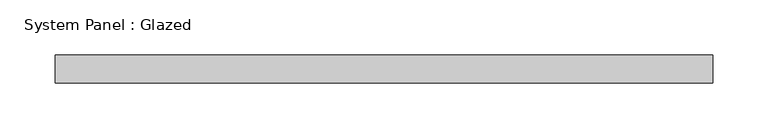
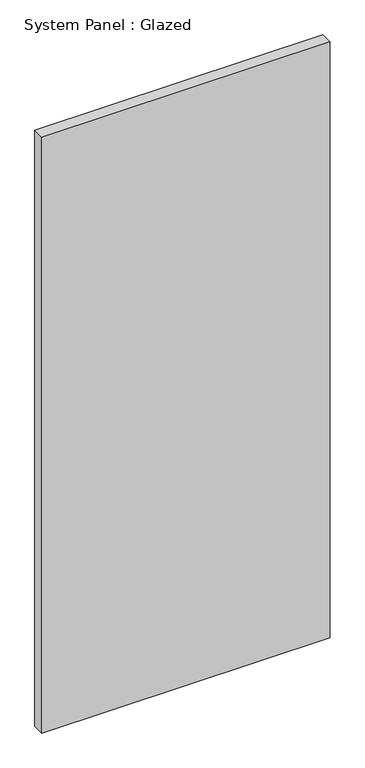
"""IFC4 building model written with IfcOpenShell, lengths in millimetres: plate geometry, System Panel : Glazed."""

from ifc_helpers import new_model, si_unit, origin, origin_with_axes, place, context, project, spatial, polyline, outline, extrude, source, transform, mapped, element, save


def system_panel_glazed_01fedee4(model_context):
    return source(origin(), model_context, "Body", "SweptSolid", [
        extrude(outline(polyline([(298.45, 19.05), (-298.45, 19.05), (-298.45, 44.45), (298.45, 44.45), (298.45, 19.05)])), origin_with_axes(), (0.0, 0.0, 1.0), 1304.017105),
    ])


if __name__ == "__main__":
    model = new_model("IFC4")
    model_context = context("Model", 3, world=origin())
    ifc_project = project(units=[si_unit("LENGTHUNIT", "METRE", prefix="MILLI")], contexts=[model_context])
    site = spatial("IfcSite", under=ifc_project)
    building = spatial("IfcBuilding", under=site)
    placement = place(None, origin())
    system_panel_glazed_shape = system_panel_glazed_01fedee4(model_context)
    element("IfcPlate", 1, ObjectType="System Panel : Glazed", at=placement, inside=building, context=model_context, shape_type="MappedRepresentation", body=[
        mapped(system_panel_glazed_shape, transform((0.0, 0.0, 0.0), x_axis=(1.0, 0.0, 0.0), y_axis=(0.0, 1.0, 0.0), z_axis=(0.0, 0.0, 1.0))),
    ])
    save(model, "model.ifc")

# Revit data of these elements
# Type "System Panel : Glazed"
#   Construction Type Id = "GSP4R"
#   Analytic Construction = "1/8 in Pilkington single glazing"
#   Visual Light Transmittance = 0.9
#   Solar Heat Gain Coefficient = 0.86
#   Heat Transfer Coefficient (U) = 1.18115 BTU/(h·ft²·°F)
#   Define Thermal Properties by = 1
# Element 1 (IfcPlate, "System Panel : Glazed")
#   Materials on its faces: "Glass"
# Materials
#   "Glass": class "Glass", colour RGB 0 128 192, transparency 0.75, Description = "Soda Lime Glass", Cost = 0
